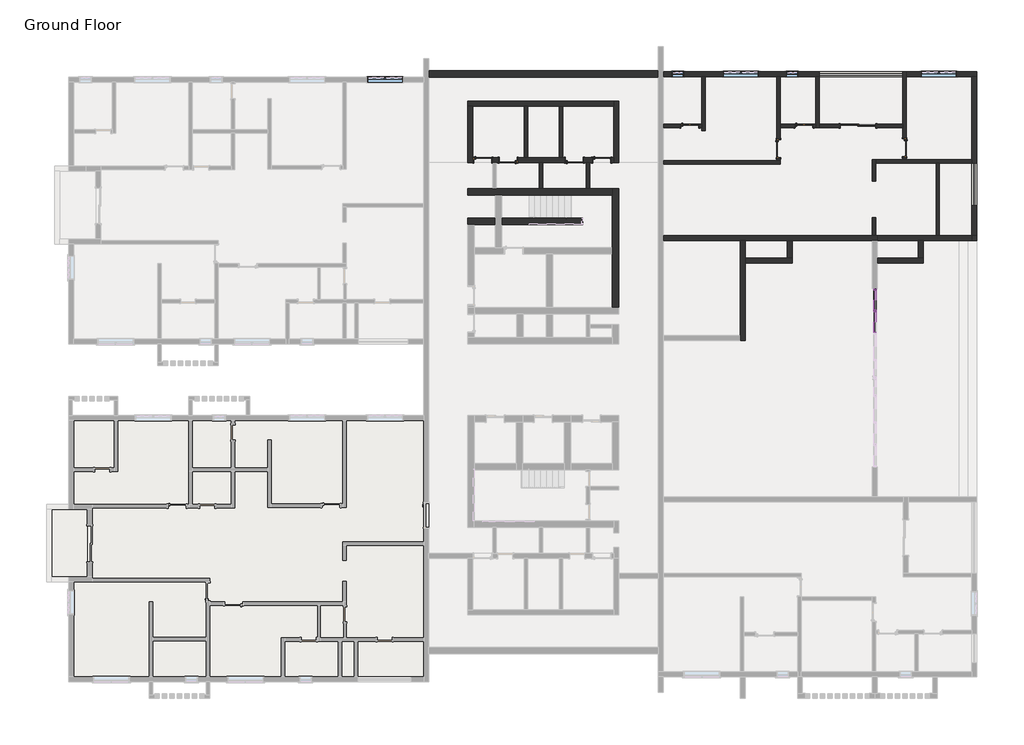
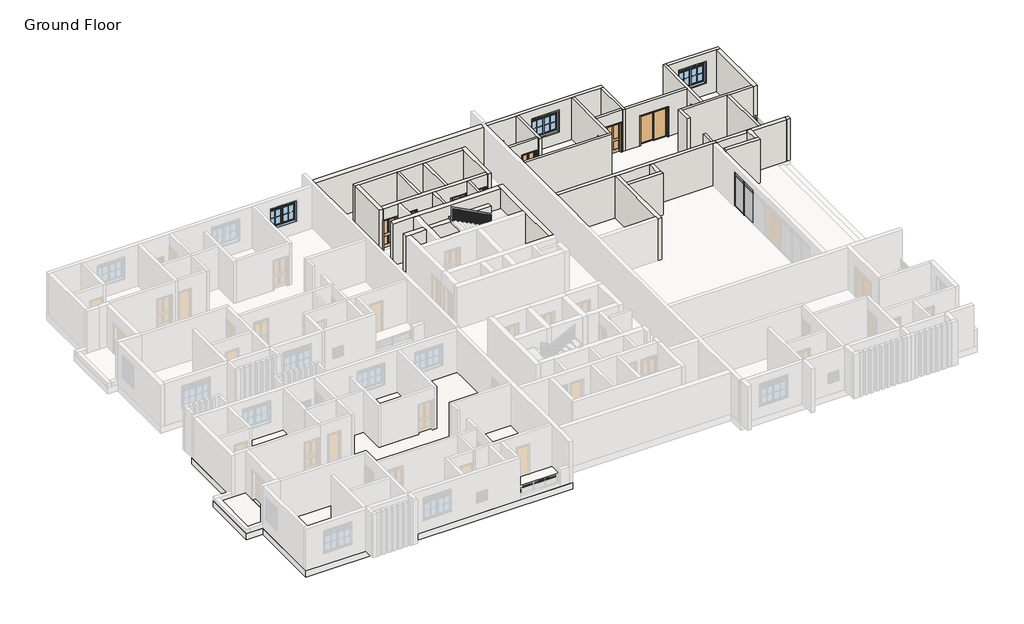
# One storey, part 5 of 9: 38 walls, 9 doors, 9 members, 5 windows, 4 plates, 2 slabs.
"""IFC4 building model written with IfcOpenShell, lengths in millimetres."""

from ifc_helpers import new_model, si_unit, frame, origin, origin_with_axes, place, context, project, spatial, polyline, outline, extrude, faceted_brep, transform, mapped, element, save
from components import door_double_sliding_6_85a7ba4d, door_interior_single_4_panel_wood_3_x_7_bed_room_doors_9f8eaeea, door_interior_single_4_panel_wood_3_x_7_bed_room_doors_167030f9, door_interior_single_4_panel_wood_3_x_7_bed_room_doors_330f8e7c, door_interior_single_4_panel_wood_3_x_7_bed_room_doors_7969a7cd, member_75d1e245, member_bf0a6844, member_74e81316, member_697f972d, member_78934672, member_3c3dc66a, member_222163d1, member_860c46db, system_panel_glazed_1d13bf28, system_panel_glazed_6ba3ac31, system_panel_glazed_eda788cd, system_panel_glazed_98578528, window_casement_double_awning_double_6_x_5_2a8633dc, window_double_hung_d0105baa

model = new_model("IFC4")

# Units and contexts
model_context = context("Model", 3, world=origin())
ifc_project = project(units=[si_unit("LENGTHUNIT", "METRE", prefix="MILLI")], contexts=[model_context])

# Site, building, storey
site = spatial("IfcSite", under=ifc_project)
building = spatial("IfcBuilding", under=site)
storey = spatial("IfcBuildingStorey", under=building, Name="Ground Floor", Elevation=0.0)

# Doors
placement = place(None, origin())
door_double_sliding_6_shape = door_double_sliding_6_85a7ba4d(model_context)
element("IfcDoor", 1, ObjectType="Door-Double-Sliding : 6'", at=placement, inside=storey, context=model_context, shape_type="MappedRepresentation", body=[
    mapped(door_double_sliding_6_shape, transform((26006.4546318, 26335.734892, 0.0), x_axis=(1.0, 0.0, 0.0), y_axis=(0.0, 1.0, 0.0), z_axis=(0.0, 0.0, 1.0))),
])
door_interior_single_4_panel_wood_3_x_7_bed_room_doors_shape = door_interior_single_4_panel_wood_3_x_7_bed_room_doors_9f8eaeea(model_context)
element("IfcDoor", 2, ObjectType="Door-Interior-Single-4_Panel-Wood : 3' x 7' Bed Room Doors", at=placement, inside=storey, context=model_context, shape_type="MappedRepresentation", body=[
    mapped(door_interior_single_4_panel_wood_3_x_7_bed_room_doors_shape, transform((17395.8546318, 26465.909892, 0.0), x_axis=(1.0, 0.0, 0.0), y_axis=(0.0, 1.0, 0.0), z_axis=(0.0, 0.0, 1.0))),
])
element("IfcDoor", 3, ObjectType="Door-Interior-Single-4_Panel-Wood : 3' x 7' Bed Room Doors", at=placement, inside=storey, context=model_context, shape_type="MappedRepresentation", body=[
    mapped(door_interior_single_4_panel_wood_3_x_7_bed_room_doors_shape, transform((23237.8546318, 26465.909892, 0.0), x_axis=(1.0, 0.0, 0.0), y_axis=(0.0, 1.0, 0.0), z_axis=(0.0, 0.0, 1.0))),
])
element("IfcDoor", 4, ObjectType="Door-Interior-Single-4_Panel-Wood : 3' x 7' Bed Room Doors", at=placement, inside=storey, context=model_context, shape_type="MappedRepresentation", body=[
    mapped(door_interior_single_4_panel_wood_3_x_7_bed_room_doors_shape, transform((28384.5296318, 25357.834892, 0.0), x_axis=(0.0, -1.0, 0.0), y_axis=(1.0, 0.0, 0.0), z_axis=(0.0, 0.0, 1.0))),
])
door_interior_single_4_panel_wood_3_x_7_bed_room_doors_2_shape = door_interior_single_4_panel_wood_3_x_7_bed_room_doors_167030f9(model_context)
element("IfcDoor", 5, ObjectType="Door-Interior-Single-4_Panel-Wood : 3' x 7' Bed Room Doors", at=placement, inside=storey, context=model_context, shape_type="MappedRepresentation", body=[
    mapped(door_interior_single_4_panel_wood_3_x_7_bed_room_doors_2_shape, transform((21926.5796318, 25307.034892, 0.0), x_axis=(0.0, -1.0, 0.0), y_axis=(1.0, 0.0, 0.0), z_axis=(0.0, 0.0, 1.0))),
])
door_interior_single_4_panel_wood_3_x_7_bed_room_doors_3_shape = door_interior_single_4_panel_wood_3_x_7_bed_room_doors_330f8e7c(model_context)
element("IfcDoor", 6, ObjectType="Door-Interior-Single-4_Panel-Wood : 3' x 7' Bed Room Doors", at=placement, inside=storey, context=model_context, shape_type="MappedRepresentation", body=[
    mapped(door_interior_single_4_panel_wood_3_x_7_bed_room_doors_3_shape, transform((8099.4546318, 24719.659892, 0.0), x_axis=(-1.0, 0.0, 0.0), y_axis=(0.0, -1.0, 0.0), z_axis=(0.0, 0.0, 1.0))),
])
element("IfcDoor", 7, ObjectType="Door-Interior-Single-4_Panel-Wood : 3' x 7' Bed Room Doors", at=placement, inside=storey, context=model_context, shape_type="MappedRepresentation", body=[
    mapped(door_interior_single_4_panel_wood_3_x_7_bed_room_doors_3_shape, transform((6804.0546318, 24726.009892, 0.0), x_axis=(1.0, 0.0, 0.0), y_axis=(0.0, 1.0, 0.0), z_axis=(0.0, 0.0, 1.0))),
])
element("IfcDoor", 8, ObjectType="Door-Interior-Single-4_Panel-Wood : 3' x 7' Bed Room Doors", at=placement, inside=storey, context=model_context, shape_type="MappedRepresentation", body=[
    mapped(door_interior_single_4_panel_wood_3_x_7_bed_room_doors_3_shape, transform((12887.3546318, 24726.009892, 0.0), x_axis=(1.0, 0.0, 0.0), y_axis=(0.0, 1.0, 0.0), z_axis=(0.0, 0.0, 1.0))),
])
door_interior_single_4_panel_wood_3_x_7_bed_room_doors_4_shape = door_interior_single_4_panel_wood_3_x_7_bed_room_doors_7969a7cd(model_context)
element("IfcDoor", 9, ObjectType="Door-Interior-Single-4_Panel-Wood : 3' x 7' Bed Room Doors", at=placement, inside=storey, context=model_context, shape_type="MappedRepresentation", body=[
    mapped(door_interior_single_4_panel_wood_3_x_7_bed_room_doors_4_shape, transform((11490.3546318, 24719.659892, 0.0), x_axis=(1.0, 0.0, 0.0), y_axis=(0.0, 1.0, 0.0), z_axis=(0.0, 0.0, 1.0))),
])

# Members
member_shape = member_75d1e245(model_context)
element("IfcMember", 10, ObjectType="Rectangular Mullion : 2.5\" x 5\" rectangular", at=placement, inside=storey, context=model_context, shape_type="MappedRepresentation", body=[
    mapped(member_shape, transform((26870.0546318, 17001.234892, 2286.0), x_axis=(0.0, 1.0, 0.0), y_axis=(1.0, 0.0, 0.0), z_axis=(0.0, 0.0, -1.0))),
])
member_2_shape = member_bf0a6844(model_context)
element("IfcMember", 11, ObjectType="Rectangular Mullion : 2.5\" x 5\" rectangular", at=placement, inside=storey, context=model_context, shape_type="MappedRepresentation", body=[
    mapped(member_2_shape, transform((26870.0546318, 16969.484892, 2286.0), x_axis=(0.0, 0.0, 1.0), y_axis=(1.0, 0.0, 0.0), z_axis=(0.0, 1.0, 0.0))),
])
member_3_shape = member_74e81316(model_context)
element("IfcMember", 12, ObjectType="Rectangular Mullion : 2.5\" x 5\" rectangular", at=placement, inside=storey, context=model_context, shape_type="MappedRepresentation", body=[
    mapped(member_3_shape, transform((26870.0546318, 16969.484892, 2590.8), x_axis=(0.0, 0.0, 1.0), y_axis=(1.0, 0.0, 0.0), z_axis=(0.0, 1.0, 0.0))),
])
member_4_shape = member_697f972d(model_context)
element("IfcMember", 13, ObjectType="Rectangular Mullion : 2.5\" x 5\" rectangular", at=placement, inside=storey, context=model_context, shape_type="MappedRepresentation", body=[
    mapped(member_4_shape, transform((26870.0546318, 18080.734892, 2286.0), x_axis=(0.0, 0.0, 1.0), y_axis=(1.0, 0.0, 0.0), z_axis=(0.0, 1.0, 0.0))),
])
member_5_shape = member_78934672(model_context)
element("IfcMember", 14, ObjectType="Rectangular Mullion : 2.5\" x 5\" rectangular", at=placement, inside=storey, context=model_context, shape_type="MappedRepresentation", body=[
    mapped(member_5_shape, transform((26870.0546318, 18080.734892, 2590.8), x_axis=(0.0, 0.0, 1.0), y_axis=(1.0, 0.0, 0.0), z_axis=(0.0, 1.0, 0.0))),
])
member_6_shape = member_3c3dc66a(model_context)
element("IfcMember", 15, ObjectType="Rectangular Mullion : 2.5\" x 5\" rectangular", at=placement, inside=storey, context=model_context, shape_type="MappedRepresentation", body=[
    mapped(member_6_shape, transform((26870.0546318, 18144.234892, 2286.0), x_axis=(0.0, 1.0, 0.0), y_axis=(1.0, 0.0, 0.0), z_axis=(0.0, 0.0, -1.0))),
])
member_7_shape = member_222163d1(model_context)
element("IfcMember", 16, ObjectType="Rectangular Mullion : 2.5\" x 5\" rectangular", at=placement, inside=storey, context=model_context, shape_type="MappedRepresentation", body=[
    mapped(member_7_shape, transform((26870.0546318, 17001.234892, 0.0), x_axis=(0.0, 1.0, 0.0), y_axis=(1.0, 0.0, 0.0), z_axis=(0.0, 0.0, -1.0))),
])
element("IfcMember", 17, ObjectType="Rectangular Mullion : 2.5\" x 5\" rectangular", at=placement, inside=storey, context=model_context, shape_type="MappedRepresentation", body=[
    mapped(member_5_shape, transform((26870.0546318, 17032.984892, 0.0), x_axis=(0.0, 0.0, -1.0), y_axis=(1.0, 0.0, 0.0), z_axis=(0.0, -1.0, 0.0))),
])
member_8_shape = member_860c46db(model_context)
element("IfcMember", 18, ObjectType="Rectangular Mullion : 2.5\" x 5\" rectangular", at=placement, inside=storey, context=model_context, shape_type="MappedRepresentation", body=[
    mapped(member_8_shape, transform((26870.0546318, 18144.234892, 0.0), x_axis=(0.0, 1.0, 0.0), y_axis=(1.0, 0.0, 0.0), z_axis=(0.0, 0.0, -1.0))),
])

# Plates
system_panel_glazed_shape = system_panel_glazed_1d13bf28(model_context)
element("IfcPlate", 19, ObjectType="System Panel : Glazed", at=placement, inside=storey, context=model_context, shape_type="MappedRepresentation", body=[
    mapped(system_panel_glazed_shape, transform((26870.0546318, 16429.734892, 2317.75), x_axis=(0.0, 1.0, 0.0), y_axis=(-1.0, 0.0, 0.0), z_axis=(0.0, 0.0, 1.0))),
])
system_panel_glazed_2_shape = system_panel_glazed_6ba3ac31(model_context)
element("IfcPlate", 20, ObjectType="System Panel : Glazed", at=placement, inside=storey, context=model_context, shape_type="MappedRepresentation", body=[
    mapped(system_panel_glazed_2_shape, transform((26870.0546318, 17556.859892, 2317.75), x_axis=(0.0, 1.0, 0.0), y_axis=(-1.0, 0.0, 0.0), z_axis=(0.0, 0.0, 1.0))),
])
system_panel_glazed_3_shape = system_panel_glazed_eda788cd(model_context)
element("IfcPlate", 21, ObjectType="System Panel : Glazed", at=placement, inside=storey, context=model_context, shape_type="MappedRepresentation", body=[
    mapped(system_panel_glazed_3_shape, transform((26870.0546318, 17556.859892, 63.5), x_axis=(0.0, 1.0, 0.0), y_axis=(-1.0, 0.0, 0.0), z_axis=(0.0, 0.0, 1.0))),
])
system_panel_glazed_4_shape = system_panel_glazed_98578528(model_context)
element("IfcPlate", 22, ObjectType="System Panel : Glazed", at=placement, inside=storey, context=model_context, shape_type="MappedRepresentation", body=[
    mapped(system_panel_glazed_4_shape, transform((26870.0546318, 16429.734892, 63.5), x_axis=(0.0, 1.0, 0.0), y_axis=(-1.0, 0.0, 0.0), z_axis=(0.0, 0.0, 1.0))),
])

# Slabs
element("IfcSlab", 23, ObjectType="Deck", at=placement, inside=storey, context=model_context, shape_type="Brep", body=[
    faceted_brep([(-14392.2453682, 7095.234892, -457.2), (-14392.2453682, 6841.234892, -457.2), (-13439.7453682, 6841.234892, -457.2), (-13439.7453682, 3386.834892, -457.2), (-14392.2453682, 3386.834892, -457.2), (-14392.2453682, 3132.834892, -457.2), (-15522.5453682, 3132.834892, -457.2), (-15522.5453682, 7095.234892, -457.2), (-14392.2453682, 7095.234892, 0.0), (-15522.5453682, 7095.234892, 0.0), (-15522.5453682, 6841.234892, 0.0), (-15522.5453682, 3132.834892, 0.0), (-15268.5453682, 3132.834892, 0.0), (-14392.2453682, 3132.834892, 0.0), (-14392.2453682, 3386.834892, 0.0), (-13439.7453682, 3386.834892, 0.0), (-13439.7453682, 6841.234892, 0.0), (-14392.2453682, 6841.234892, 0.0)], [[[0, 1, 2, 3, 4, 5, 6, 7]], [[8, 9, 10, 11, 12, 13, 14, 15, 16, 17]], [[1, 0, 8, 17]], [[2, 1, 17, 16]], [[3, 2, 16, 15]], [[4, 3, 15, 14]], [[5, 4, 14, 13]], [[6, 5, 13, 12, 11]], [[7, 6, 11, 10, 9]], [[0, 7, 9, 8]]]),
])
element("IfcSlab", 24, ObjectType="cream", at=placement, inside=storey, context=model_context, shape_type="Brep", body=[
    faceted_brep([(4035.4546318, 11641.834892, -457.2), (4035.4546318, -1997.965108, -457.2), (-14392.2453682, -1997.965108, -457.2), (-14392.2453682, 3386.834892, -457.2), (-13439.7453682, 3386.834892, -457.2), (-13439.7453682, 6841.234892, -457.2), (-14392.2453682, 6841.234892, -457.2), (-14392.2453682, 11641.834892, -457.2), (4035.4546318, 11641.834892, 0.0), (3781.4546318, 11641.834892, 0.0), (-14392.2453682, 11641.834892, 0.0), (-14392.2453682, 11387.834892, 0.0), (-14392.2453682, 6841.234892, 0.0), (-14138.2453682, 6841.234892, 0.0), (-13439.7453682, 6841.234892, 0.0), (-13439.7453682, 5990.334892, 0.0), (-13439.7453682, 4161.534892, 0.0), (-13439.7453682, 3386.834892, 0.0), (-14392.2453682, 3386.834892, 0.0), (-14392.2453682, 3132.834892, 0.0), (-14392.2453682, -1743.965108, 0.0), (-14392.2453682, -1997.965108, 0.0), (403.2546318, -1997.965108, 0.0), (3146.4546318, -1997.965108, 0.0), (3781.4546318, -1997.965108, 0.0), (4035.4546318, -1997.965108, 0.0), (4035.4546318, 5901.434892, 0.0), (4035.4546318, 7171.434892, 0.0)], [[[0, 1, 2, 3, 4, 5, 6, 7]], [[8, 9, 10, 11, 12, 13, 14, 15, 16, 17, 18, 19, 20, 21, 22, 23, 24, 25, 26, 27]], [[1, 0, 8, 27, 26, 25]], [[2, 1, 25, 24, 23, 22, 21]], [[3, 2, 21, 20, 19, 18]], [[4, 3, 18, 17]], [[5, 4, 17, 16, 15, 14]], [[6, 5, 14, 13, 12]], [[7, 6, 12, 11, 10]], [[0, 7, 10, 9, 8]]]),
])

# Walls
element("IfcWall", 25, ObjectType="12\" EXTERIOR WALL", at=placement, inside=storey, context=model_context, shape_type="Brep", body=[
    faceted_brep([(13763.6546318, 17179.034892, 0.0), (13763.6546318, 23249.634892, 0.0), (13763.6546318, 23249.634892, 3048.0), (13763.6546318, 17179.034892, 3048.0), (13433.4546318, 23249.634892, 0.0), (13433.4546318, 22919.434892, 0.0), (13433.4546318, 20252.434892, 0.0), (13433.4546318, 19922.234892, 0.0), (13433.4546318, 17179.034892, 0.0), (13433.4546318, 17179.034892, 3048.0), (13433.4546318, 20252.434892, 3048.0), (13433.4546318, 22919.434892, 3048.0), (13433.4546318, 23249.634892, 3048.0)], [[[0, 1, 2, 3]], [[4, 5, 6, 7, 8, 9, 10, 11, 12]], [[1, 0, 8, 7, 6, 5, 4]], [[8, 0, 3, 9]], [[1, 4, 12, 2]], [[3, 2, 12, 11, 10, 9]]]),
])
element("IfcWall", 26, ObjectType="12\" EXTERIOR WALL", at=placement, inside=storey, context=model_context, shape_type="Brep", body=[
    faceted_brep([(13433.4546318, 23249.634892, 0.0), (12265.0546318, 23249.634892, 0.0), (12087.2546318, 23249.634892, 0.0), (9877.4546318, 23249.634892, 0.0), (9699.6546318, 23249.634892, 0.0), (7489.8546318, 23249.634892, 0.0), (7312.0546318, 23249.634892, 0.0), (6042.0546318, 23249.634892, 0.0), (6042.0546318, 23249.634892, 3048.0), (7312.0546318, 23249.634892, 3048.0), (7489.8546318, 23249.634892, 3048.0), (9699.6546318, 23249.634892, 3048.0), (9877.4546318, 23249.634892, 3048.0), (12087.2546318, 23249.634892, 3048.0), (12265.0546318, 23249.634892, 3048.0), (13433.4546318, 23249.634892, 3048.0), (6042.0546318, 22919.434892, 0.0), (7439.0546318, 22919.434892, 0.0), (7769.2546318, 22919.434892, 0.0), (13433.4546318, 22919.434892, 0.0), (13433.4546318, 22919.434892, 3048.0), (9166.2546318, 22919.434892, 3048.0), (7769.2546318, 22919.434892, 3048.0), (7439.0546318, 22919.434892, 3048.0), (6042.0546318, 22919.434892, 3048.0)], [[[0, 1, 2, 3, 4, 5, 6, 7, 8, 9, 10, 11, 12, 13, 14, 15]], [[16, 17, 18, 19, 20, 21, 22, 23, 24]], [[7, 6, 5, 4, 3, 2, 1, 0, 19, 18, 17, 16]], [[7, 16, 24, 8]], [[19, 0, 15, 20]], [[15, 14, 13, 12, 11, 10, 9, 8, 24, 23, 22, 21, 20]]]),
])
element("IfcWall", 27, ObjectType="12\" EXTERIOR WALL", at=placement, inside=storey, context=model_context, shape_type="Brep", body=[
    faceted_brep([(4035.4546318, 28964.634892, 0.0), (15770.2546318, 28964.634892, 0.0), (15770.2546318, 28964.634892, 3048.0), (4035.4546318, 28964.634892, 3048.0), (15770.2546318, 29294.834892, 0.0), (4035.4546318, 29294.834892, 0.0), (4035.4546318, 29294.834892, 3048.0), (15770.2546318, 29294.834892, 3048.0), (15770.2546318, 29244.034892, 3048.0)], [[[0, 1, 2, 3]], [[4, 5, 6, 7]], [[1, 0, 5, 4]], [[5, 0, 3, 6]], [[1, 4, 7, 8, 2]], [[3, 2, 8, 7, 6]]]),
])
element("IfcWall", 28, ObjectType="12\" EXTERIOR WALL", at=placement, inside=storey, context=model_context, shape_type="Brep", body=[
    faceted_brep([(11909.4546318, 21751.034892, 3200.4), (11909.4546318, 21751.034892, 0.0), (7769.2546318, 21751.034892, 0.0), (7769.2546318, 21751.034892, 3048.0), (9166.2546318, 21751.034892, 3048.0), (9166.2546318, 21751.034892, 3200.4), (11909.4546318, 21420.834892, 0.0), (11909.4546318, 21420.834892, 3200.4), (9166.2546318, 21420.834892, 3200.4), (9166.2546318, 21420.834892, 3048.0), (7769.2546318, 21420.834892, 3048.0), (7769.2546318, 21420.834892, 0.0)], [[[0, 1, 2, 3, 4, 5]], [[6, 7, 8, 9, 10, 11]], [[1, 6, 11, 2]], [[7, 0, 5, 8]], [[1, 0, 7, 6]], [[9, 4, 3, 10]], [[4, 9, 8, 5]], [[3, 2, 11, 10]]]),
    faceted_brep([(6042.0546318, 21751.034892, 0.0), (6042.0546318, 21751.034892, 3048.0), (7439.0546318, 21751.034892, 3048.0), (7439.0546318, 21751.034892, 0.0), (6042.0546318, 21420.834892, 3048.0), (6042.0546318, 21420.834892, 0.0), (6372.2546318, 21420.834892, 0.0), (7439.0546318, 21420.834892, 0.0), (7439.0546318, 21420.834892, 3048.0), (6372.2546318, 21420.834892, 3048.0)], [[[0, 1, 2, 3]], [[4, 5, 6, 7, 8, 9]], [[5, 0, 3, 7, 6]], [[0, 5, 4, 1]], [[1, 4, 9, 8, 2]], [[3, 2, 8, 7]]]),
])
element("IfcWall", 29, ObjectType="6\" INTERIOR WALL", at=placement, inside=storey, context=model_context, shape_type="SweptSolid", body=[
    extrude(outline(polyline([(9877.4546318, 24595.834892), (9877.4546318, 23249.634892), (9699.6546318, 23249.634892), (9699.6546318, 24595.834892), (9877.4546318, 24595.834892)])), origin_with_axes(), (0.0, 0.0, 1.0), 3048.0),
])
element("IfcWall", 30, ObjectType="6\" INTERIOR WALL", at=placement, inside=storey, context=model_context, shape_type="SweptSolid", body=[
    extrude(outline(polyline([(12265.0546318, 24595.834892), (12265.0546318, 23249.634892), (12087.2546318, 23249.634892), (12087.2546318, 24595.834892), (12265.0546318, 24595.834892)])), origin_with_axes(), (0.0, 0.0, 1.0), 3048.0),
])
element("IfcWall", 31, ObjectType="6\" INTERIOR WALL", at=placement, inside=storey, context=model_context, shape_type="SweptSolid", body=[
    extrude(outline(polyline([(10715.6546318, 24849.834892), (10715.6546318, 27491.434892), (10893.4546318, 27491.434892), (10893.4546318, 24849.834892), (10715.6546318, 24849.834892)])), origin_with_axes(), (0.0, 0.0, 1.0), 3048.0),
])
element("IfcWall", 32, ObjectType="6\" INTERIOR WALL", at=placement, inside=storey, context=model_context, shape_type="SweptSolid", body=[
    extrude(outline(polyline([(9090.0546318, 27491.434892), (9090.0546318, 24849.834892), (8912.2546318, 24849.834892), (8912.2546318, 27491.434892), (9090.0546318, 27491.434892)])), origin_with_axes(), (0.0, 0.0, 1.0), 3048.0),
])
element("IfcWall", 33, ObjectType="6\" INTERIOR WALL", at=placement, inside=storey, context=model_context, shape_type="Brep", body=[
    faceted_brep([(16024.2546318, 24519.634892, 0.0), (22018.6546318, 24519.634892, 0.0), (22018.6546318, 24519.634892, 3048.0), (16024.2546318, 24519.634892, 3048.0), (22018.6546318, 24697.434892, 0.0), (21840.8546318, 24697.434892, 0.0), (16024.2546318, 24697.434892, 0.0), (16024.2546318, 24697.434892, 3048.0), (21840.8546318, 24697.434892, 3048.0), (22018.6546318, 24697.434892, 3048.0)], [[[0, 1, 2, 3]], [[4, 5, 6, 7, 8, 9]], [[1, 0, 6, 5, 4]], [[6, 0, 3, 7]], [[1, 4, 9, 2]], [[3, 2, 9, 8, 7]]]),
])
element("IfcWall", 34, ObjectType="6\" INTERIOR WALL", at=placement, inside=storey, context=model_context, shape_type="SweptSolid", body=[
    extrude(outline(polyline([(0.0, 17878.4546318), (0.0, 18005.4546318), (3048.0, 18005.4546318), (3048.0, 16024.2546318), (0.0, 16024.2546318), (0.0, 16913.2546318), (2159.0, 16913.2546318), (2159.0, 17878.4546318), (0.0, 17878.4546318)])), frame((0.0, 26373.834892, 0.0), z_axis=(0.0, 1.0, 0.0), x_axis=(0.0, 0.0, 1.0)), (0.0, 0.0, 1.0), 177.8),
])
element("IfcWall", 35, ObjectType="6\" INTERIOR WALL", at=placement, inside=storey, context=model_context, shape_type="Brep", body=[
    faceted_brep([(18005.4546318, 28990.034892, 0.0), (18005.4546318, 26551.634892, 0.0), (18005.4546318, 26373.834892, 0.0), (18005.4546318, 26221.434892, 0.0), (18005.4546318, 26221.434892, 3048.0), (18005.4546318, 26373.834892, 3048.0), (18005.4546318, 26551.634892, 3048.0), (18005.4546318, 28990.034892, 3048.0), (18183.2546318, 26221.434892, 0.0), (18183.2546318, 28990.034892, 0.0), (18183.2546318, 28990.034892, 3048.0), (18183.2546318, 26221.434892, 3048.0)], [[[0, 1, 2, 3, 4, 5, 6, 7]], [[8, 9, 10, 11]], [[3, 2, 1, 0, 9, 8]], [[3, 8, 11, 4]], [[9, 0, 7, 10]], [[7, 6, 5, 4, 11, 10]]]),
])
element("IfcWall", 36, ObjectType="6\" INTERIOR WALL", at=placement, inside=storey, context=model_context, shape_type="Brep", body=[
    faceted_brep([(21840.8546318, 24824.434892, 0.0), (21840.8546318, 24697.434892, 0.0), (21840.8546318, 24697.434892, 3048.0), (21840.8546318, 28990.034892, 3048.0), (21840.8546318, 28990.034892, 0.0), (21840.8546318, 25789.634892, 0.0), (21840.8546318, 25789.634892, 2159.0), (21840.8546318, 24824.434892, 2159.0), (22018.6546318, 24697.434892, 0.0), (22018.6546318, 24824.434892, 0.0), (22018.6546318, 24824.434892, 2159.0), (22018.6546318, 25789.634892, 2159.0), (22018.6546318, 25789.634892, 0.0), (22018.6546318, 26373.834892, 0.0), (22018.6546318, 26551.634892, 0.0), (22018.6546318, 28990.034892, 0.0), (22018.6546318, 28990.034892, 3048.0), (22018.6546318, 26551.634892, 3048.0), (22018.6546318, 26373.834892, 3048.0), (22018.6546318, 24697.434892, 3048.0)], [[[0, 1, 2, 3, 4, 5, 6, 7]], [[8, 9, 10, 11, 12, 13, 14, 15, 16, 17, 18, 19]], [[4, 15, 14, 13, 12, 5]], [[8, 1, 0, 9]], [[15, 4, 3, 16]], [[1, 8, 19, 2]], [[3, 2, 19, 18, 17, 16]], [[7, 10, 9, 0]], [[10, 7, 6, 11]], [[11, 6, 5, 12]]]),
])
element("IfcWall", 37, ObjectType="6\" INTERIOR WALL", at=placement, inside=storey, context=model_context, shape_type="Brep", body=[
    faceted_brep([(23847.4546318, 28990.034892, 0.0), (23847.4546318, 26551.634892, 0.0), (23847.4546318, 26373.834892, 0.0), (23847.4546318, 26373.834892, 3048.0), (23847.4546318, 26551.634892, 3048.0), (23847.4546318, 28990.034892, 3048.0), (24025.2546318, 26373.834892, 0.0), (24025.2546318, 26551.634892, 0.0), (24025.2546318, 28990.034892, 0.0), (24025.2546318, 28990.034892, 3048.0), (24025.2546318, 26551.634892, 3048.0), (24025.2546318, 26373.834892, 3048.0)], [[[0, 1, 2, 3, 4, 5]], [[6, 7, 8, 9, 10, 11]], [[2, 1, 0, 8, 7, 6]], [[2, 6, 11, 3]], [[8, 0, 5, 9]], [[5, 4, 3, 11, 10, 9]]]),
])
element("IfcWall", 38, ObjectType="6\" INTERIOR WALL", at=placement, inside=storey, context=model_context, shape_type="SweptSolid", body=[
    extrude(outline(polyline([(0.0, 23720.4546318), (0.0, 23847.4546318), (3048.0, 23847.4546318), (3048.0, 22018.6546318), (0.0, 22018.6546318), (0.0, 22755.2546318), (2159.0, 22755.2546318), (2159.0, 23720.4546318), (0.0, 23720.4546318)])), frame((0.0, 26373.834892, 0.0), z_axis=(0.0, 1.0, 0.0), x_axis=(0.0, 0.0, 1.0)), (0.0, 0.0, 1.0), 177.8),
])
element("IfcWall", 39, ObjectType="6\" INTERIOR WALL", at=placement, inside=storey, context=model_context, shape_type="SweptSolid", body=[
    extrude(outline(polyline([(0.0, 25092.0546318), (2133.6, 25092.0546318), (2133.6, 26920.8546318), (0.0, 26920.8546318), (0.0, 28292.4546318), (3048.0, 28292.4546318), (3048.0, 24025.2546318), (0.0, 24025.2546318), (0.0, 25092.0546318)])), frame((0.0, 26373.834892, 0.0), z_axis=(0.0, 1.0, 0.0), x_axis=(0.0, 0.0, 1.0)), (0.0, 0.0, 1.0), 177.8),
])
element("IfcWall", 40, ObjectType="6\" INTERIOR WALL", at=placement, inside=storey, context=model_context, shape_type="Brep", body=[
    faceted_brep([(28470.2546318, 24748.234892, 0.0), (28470.2546318, 24875.234892, 0.0), (28470.2546318, 24875.234892, 2159.0), (28470.2546318, 25840.434892, 2159.0), (28470.2546318, 25840.434892, 0.0), (28470.2546318, 28990.034892, 0.0), (28470.2546318, 29244.034892, 0.0), (28470.2546318, 29244.034892, 3048.0), (28470.2546318, 28990.034892, 3048.0), (28470.2546318, 24748.234892, 3048.0), (28292.4546318, 24875.234892, 0.0), (28292.4546318, 24748.234892, 0.0), (28292.4546318, 24748.234892, 3048.0), (28292.4546318, 26373.834892, 3048.0), (28292.4546318, 26551.634892, 3048.0), (28292.4546318, 29244.034892, 3048.0), (28292.4546318, 29244.034892, 304.8), (28292.4546318, 29244.034892, 0.0), (28292.4546318, 28990.034892, 0.0), (28292.4546318, 26551.634892, 0.0), (28292.4546318, 26373.834892, 0.0), (28292.4546318, 25840.434892, 0.0), (28292.4546318, 25840.434892, 2159.0), (28292.4546318, 24875.234892, 2159.0)], [[[0, 1, 2, 3, 4, 5, 6, 7, 8, 9]], [[10, 11, 12, 13, 14, 15, 16, 17, 18, 19, 20, 21, 22, 23]], [[17, 6, 5, 4, 21, 20, 19, 18]], [[0, 11, 10, 1]], [[6, 17, 16, 15, 7]], [[9, 8, 7, 15, 14, 13, 12]], [[11, 0, 9, 12]], [[23, 2, 1, 10]], [[2, 23, 22, 3]], [[3, 22, 21, 4]]]),
])
element("IfcWall", 41, ObjectType="6\" INTERIOR WALL", at=placement, inside=storey, context=model_context, shape_type="Brep", body=[
    faceted_brep([(31823.0546318, 24748.234892, 0.0), (28470.2546318, 24748.234892, 0.0), (28292.4546318, 24748.234892, 0.0), (26920.8546318, 24748.234892, 0.0), (26920.8546318, 24748.234892, 3048.0), (28292.4546318, 24748.234892, 3048.0), (28470.2546318, 24748.234892, 3048.0), (31823.0546318, 24748.234892, 3048.0), (26920.8546318, 24570.434892, 0.0), (29994.2546318, 24570.434892, 0.0), (30172.0546318, 24570.434892, 0.0), (31823.0546318, 24570.434892, 0.0), (31823.0546318, 24570.434892, 3048.0), (30172.0546318, 24570.434892, 3048.0), (29994.2546318, 24570.434892, 3048.0), (26920.8546318, 24570.434892, 3048.0)], [[[0, 1, 2, 3, 4, 5, 6, 7]], [[8, 9, 10, 11, 12, 13, 14, 15]], [[3, 2, 1, 0, 11, 10, 9, 8]], [[3, 8, 15, 4]], [[7, 6, 5, 4, 15, 14, 13, 12]], [[11, 0, 7, 12]]]),
])
element("IfcWall", 42, ObjectType="6\" INTERIOR WALL", at=placement, inside=storey, context=model_context, shape_type="SweptSolid", body=[
    extrude(outline(polyline([(29994.2546318, 20862.034892), (29994.2546318, 24570.434892), (30172.0546318, 24570.434892), (30172.0546318, 20862.034892), (29994.2546318, 20862.034892)])), origin_with_axes(), (0.0, 0.0, 1.0), 3048.0),
])
element("IfcWall", 43, ObjectType="6\" INTERIOR WALL", at=placement, inside=storey, context=model_context, shape_type="Brep", body=[
    faceted_brep([(26743.0546318, 24748.234892, 0.0), (26743.0546318, 23656.034892, 0.0), (26743.0546318, 23656.034892, 3048.0), (26743.0546318, 24748.234892, 3048.0), (26920.8546318, 23656.034892, 0.0), (26920.8546318, 24570.434892, 0.0), (26920.8546318, 24748.234892, 0.0), (26920.8546318, 24748.234892, 3048.0), (26920.8546318, 24570.434892, 3048.0), (26920.8546318, 23656.034892, 3048.0)], [[[0, 1, 2, 3]], [[4, 5, 6, 7, 8, 9]], [[1, 0, 6, 5, 4]], [[1, 4, 9, 2]], [[6, 0, 3, 7]], [[3, 2, 9, 8, 7]]]),
])
element("IfcWall", 44, ObjectType="6\" INTERIOR WALL", at=placement, inside=storey, context=model_context, shape_type="SweptSolid", body=[
    extrude(outline(polyline([(26920.8546318, 21776.434892), (26920.8546318, 20862.034892), (26743.0546318, 20862.034892), (26743.0546318, 21776.434892), (26920.8546318, 21776.434892)])), origin_with_axes(), (0.0, 0.0, 1.0), 3048.0),
])
element("IfcWall", 45, ObjectType="9\" EXTERIOR WALL", at=placement, inside=storey, context=model_context, shape_type="Brep", body=[
    faceted_brep([(13763.6546318, 24595.834892, 0.0), (13763.6546318, 27745.434892, 0.0), (13763.6546318, 27745.434892, 3048.0), (13763.6546318, 24595.834892, 3048.0), (13509.6546318, 27745.434892, 0.0), (13509.6546318, 27491.434892, 0.0), (13509.6546318, 24849.834892, 0.0), (13509.6546318, 24595.834892, 0.0), (13509.6546318, 24595.834892, 3048.0), (13509.6546318, 27745.434892, 3048.0)], [[[0, 1, 2, 3]], [[4, 5, 6, 7, 8, 9]], [[1, 0, 7, 6, 5, 4]], [[1, 4, 9, 2]], [[7, 0, 3, 8]], [[3, 2, 9, 8]]]),
])
element("IfcWall", 46, ObjectType="9\" EXTERIOR WALL", at=placement, inside=storey, context=model_context, shape_type="Brep", body=[
    faceted_brep([(13509.6546318, 27745.434892, 0.0), (6042.0546318, 27745.434892, 0.0), (6042.0546318, 27745.434892, 3048.0), (13509.6546318, 27745.434892, 3048.0), (6042.0546318, 27491.434892, 0.0), (6296.0546318, 27491.434892, 0.0), (8912.2546318, 27491.434892, 0.0), (9090.0546318, 27491.434892, 0.0), (10715.6546318, 27491.434892, 0.0), (10893.4546318, 27491.434892, 0.0), (13509.6546318, 27491.434892, 0.0), (13509.6546318, 27491.434892, 3048.0), (6042.0546318, 27491.434892, 3048.0)], [[[0, 1, 2, 3]], [[4, 5, 6, 7, 8, 9, 10, 11, 12]], [[1, 0, 10, 9, 8, 7, 6, 5, 4]], [[10, 0, 3, 11]], [[1, 4, 12, 2]], [[3, 2, 12, 11]]]),
])
element("IfcWall", 47, ObjectType="9\" EXTERIOR WALL", at=placement, inside=storey, context=model_context, shape_type="Brep", body=[
    faceted_brep([(6296.0546318, 24595.834892, 0.0), (6296.0546318, 24849.834892, 0.0), (6296.0546318, 27491.434892, 0.0), (6296.0546318, 27491.434892, 3048.0), (6296.0546318, 24849.834892, 3048.0), (6296.0546318, 24595.834892, 3048.0), (6042.0546318, 27491.434892, 0.0), (6042.0546318, 24595.834892, 0.0), (6042.0546318, 24595.834892, 3048.0), (6042.0546318, 27491.434892, 3048.0)], [[[0, 1, 2, 3, 4, 5]], [[6, 7, 8, 9]], [[2, 1, 0, 7, 6]], [[2, 6, 9, 3]], [[7, 0, 5, 8]], [[5, 4, 3, 9, 8]]]),
])
element("IfcWall", 48, ObjectType="9\" EXTERIOR WALL", at=placement, inside=storey, context=model_context, shape_type="Brep", body=[
    faceted_brep([(7616.8546318, 24595.834892, 0.0), (7616.8546318, 24595.834892, 2159.0), (8582.0546318, 24595.834892, 2159.0), (8582.0546318, 24595.834892, 0.0), (9699.6546318, 24595.834892, 0.0), (9877.4546318, 24595.834892, 0.0), (11007.7546318, 24595.834892, 0.0), (11007.7546318, 24595.834892, 2159.0), (11972.9546318, 24595.834892, 2159.0), (11972.9546318, 24595.834892, 0.0), (12087.2546318, 24595.834892, 0.0), (12265.0546318, 24595.834892, 0.0), (12404.7546318, 24595.834892, 0.0), (12404.7546318, 24595.834892, 2159.0), (13369.9546318, 24595.834892, 2159.0), (13369.9546318, 24595.834892, 0.0), (13509.6546318, 24595.834892, 0.0), (13509.6546318, 24595.834892, 3048.0), (12265.0546318, 24595.834892, 3048.0), (12087.2546318, 24595.834892, 3048.0), (9877.4546318, 24595.834892, 3048.0), (9699.6546318, 24595.834892, 3048.0), (7489.8546318, 24595.834892, 3048.0), (7312.0546318, 24595.834892, 3048.0), (6296.0546318, 24595.834892, 3048.0), (6296.0546318, 24595.834892, 0.0), (6321.4546318, 24595.834892, 0.0), (6321.4546318, 24595.834892, 2159.0), (7286.6546318, 24595.834892, 2159.0), (7286.6546318, 24595.834892, 0.0), (7312.0546318, 24595.834892, 0.0), (7489.8546318, 24595.834892, 0.0), (7616.8546318, 24849.834892, 2159.0), (7616.8546318, 24849.834892, 0.0), (7286.6546318, 24849.834892, 0.0), (7286.6546318, 24849.834892, 2159.0), (6321.4546318, 24849.834892, 2159.0), (6321.4546318, 24849.834892, 0.0), (6296.0546318, 24849.834892, 0.0), (6296.0546318, 24849.834892, 3048.0), (8912.2546318, 24849.834892, 3048.0), (9090.0546318, 24849.834892, 3048.0), (10715.6546318, 24849.834892, 3048.0), (10893.4546318, 24849.834892, 3048.0), (13509.6546318, 24849.834892, 3048.0), (13509.6546318, 24849.834892, 0.0), (13369.9546318, 24849.834892, 0.0), (13369.9546318, 24849.834892, 2159.0), (12404.7546318, 24849.834892, 2159.0), (12404.7546318, 24849.834892, 0.0), (11972.9546318, 24849.834892, 0.0), (11972.9546318, 24849.834892, 2159.0), (11007.7546318, 24849.834892, 2159.0), (11007.7546318, 24849.834892, 0.0), (10893.4546318, 24849.834892, 0.0), (10715.6546318, 24849.834892, 0.0), (9090.0546318, 24849.834892, 0.0), (8912.2546318, 24849.834892, 0.0), (8582.0546318, 24849.834892, 0.0), (8582.0546318, 24849.834892, 2159.0)], [[[0, 1, 2, 3, 4, 5, 6, 7, 8, 9, 10, 11, 12, 13, 14, 15, 16, 17, 18, 19, 20, 21, 22, 23, 24, 25, 26, 27, 28, 29, 30, 31]], [[32, 33, 34, 35, 36, 37, 38, 39, 40, 41, 42, 43, 44, 45, 46, 47, 48, 49, 50, 51, 52, 53, 54, 55, 56, 57, 58, 59]], [[25, 38, 37, 26]], [[45, 16, 15, 46]], [[33, 0, 31, 30, 29, 34]], [[3, 58, 57, 56, 55, 54, 53, 6, 5, 4]], [[9, 50, 49, 12, 11, 10]], [[16, 45, 44, 17]], [[38, 25, 24, 39]], [[24, 23, 22, 21, 20, 19, 18, 17, 44, 43, 42, 41, 40, 39]], [[32, 1, 0, 33]], [[1, 32, 59, 2]], [[2, 59, 58, 3]], [[8, 51, 50, 9]], [[51, 8, 7, 52]], [[52, 7, 6, 53]], [[28, 35, 34, 29]], [[35, 28, 27, 36]], [[36, 27, 26, 37]], [[14, 47, 46, 15]], [[47, 14, 13, 48]], [[48, 13, 12, 49]]]),
])
element("IfcWall", 49, ObjectType="9\" EXTERIOR WALL", at=placement, inside=storey, context=model_context, shape_type="Brep", body=[
    faceted_brep([(16024.2546318, 20608.034892, 0.0), (19986.6546318, 20608.034892, 0.0), (20240.6546318, 20608.034892, 0.0), (22374.2546318, 20608.034892, 0.0), (22628.2546318, 20608.034892, 0.0), (26743.0546318, 20608.034892, 0.0), (26997.0546318, 20608.034892, 0.0), (26997.0546318, 20608.034892, 3048.0), (26743.0546318, 20608.034892, 3048.0), (22628.2546318, 20608.034892, 3048.0), (22374.2546318, 20608.034892, 3048.0), (20240.6546318, 20608.034892, 3048.0), (19986.6546318, 20608.034892, 3048.0), (16024.2546318, 20608.034892, 3048.0), (26997.0546318, 20862.034892, 0.0), (26920.8546318, 20862.034892, 0.0), (26743.0546318, 20862.034892, 0.0), (16024.2546318, 20862.034892, 0.0), (16024.2546318, 20862.034892, 3048.0), (26743.0546318, 20862.034892, 3048.0), (26920.8546318, 20862.034892, 3048.0), (26997.0546318, 20862.034892, 3048.0)], [[[0, 1, 2, 3, 4, 5, 6, 7, 8, 9, 10, 11, 12, 13]], [[14, 15, 16, 17, 18, 19, 20, 21]], [[6, 5, 4, 3, 2, 1, 0, 17, 16, 15, 14]], [[17, 0, 13, 18]], [[6, 14, 21, 7]], [[13, 12, 11, 10, 9, 8, 7, 21, 20, 19, 18]]]),
])
element("IfcWall", 50, ObjectType="9\" EXTERIOR WALL", at=placement, inside=storey, context=model_context, shape_type="Brep", body=[
    faceted_brep([(19986.6546318, 20608.034892, 0.0), (19986.6546318, 15731.234892, 0.0), (19986.6546318, 15477.234892, 0.0), (19986.6546318, 15477.234892, 3048.0), (19986.6546318, 20608.034892, 3048.0), (20240.6546318, 15477.234892, 0.0), (20240.6546318, 19439.634892, 0.0), (20240.6546318, 19693.634892, 0.0), (20240.6546318, 20608.034892, 0.0), (20240.6546318, 20608.034892, 3048.0), (20240.6546318, 19693.634892, 3048.0), (20240.6546318, 19439.634892, 3048.0), (20240.6546318, 15477.234892, 3048.0)], [[[0, 1, 2, 3, 4]], [[5, 6, 7, 8, 9, 10, 11, 12]], [[2, 1, 0, 8, 7, 6, 5]], [[8, 0, 4, 9]], [[2, 5, 12, 3]], [[4, 3, 12, 11, 10, 9]]]),
])
element("IfcWall", 51, ObjectType="9\" EXTERIOR WALL", at=placement, inside=storey, context=model_context, shape_type="Brep", body=[
    faceted_brep([(20240.6546318, 19439.634892, 0.0), (22628.2546318, 19439.634892, 0.0), (22628.2546318, 19439.634892, 3048.0), (20240.6546318, 19439.634892, 3048.0), (22628.2546318, 19693.634892, 0.0), (22374.2546318, 19693.634892, 0.0), (20240.6546318, 19693.634892, 0.0), (20240.6546318, 19693.634892, 3048.0), (22628.2546318, 19693.634892, 3048.0)], [[[0, 1, 2, 3]], [[4, 5, 6, 7, 8]], [[1, 0, 6, 5, 4]], [[6, 0, 3, 7]], [[1, 4, 8, 2]], [[3, 2, 8, 7]]]),
])
element("IfcWall", 52, ObjectType="9\" EXTERIOR WALL", at=placement, inside=storey, context=model_context, shape_type="SweptSolid", body=[
    extrude(outline(polyline([(22628.2546318, 20608.034892), (22628.2546318, 19693.634892), (22374.2546318, 19693.634892), (22374.2546318, 20608.034892), (22628.2546318, 20608.034892)])), origin_with_axes(), (0.0, 0.0, 1.0), 3048.0),
])
element("IfcWall", 53, ObjectType="9\" EXTERIOR WALL", at=placement, inside=storey, context=model_context, shape_type="Brep", body=[
    faceted_brep([(26997.0546318, 19439.634892, 0.0), (29333.8546318, 19439.634892, 0.0), (29333.8546318, 19439.634892, 3200.4), (26997.0546318, 19439.634892, 3200.4), (26997.0546318, 19693.634892, 0.0), (26997.0546318, 19693.634892, 3200.4), (29079.8546318, 19693.634892, 3200.4), (29333.8546318, 19693.634892, 3200.4), (29333.8546318, 19693.634892, 0.0), (29079.8546318, 19693.634892, 0.0)], [[[0, 1, 2, 3]], [[4, 5, 6, 7, 8, 9]], [[1, 0, 4, 9, 8]], [[3, 2, 7, 6, 5]], [[2, 1, 8, 7]], [[0, 3, 5, 4]]]),
])
element("IfcWall", 54, ObjectType="9\" EXTERIOR WALL", at=placement, inside=storey, context=model_context, shape_type="SweptSolid", body=[
    extrude(outline(polyline([(29333.8546318, 20608.034892), (29333.8546318, 19693.634892), (29079.8546318, 19693.634892), (29079.8546318, 20608.034892), (29333.8546318, 20608.034892)])), origin_with_axes(), (0.0, 0.0, 1.0), 3200.4),
])
element("IfcWall", 55, ObjectType="9\" EXTERIOR WALL", at=placement, inside=storey, context=model_context, shape_type="Brep", body=[
    faceted_brep([(16024.2546318, 28990.034892, 0.0), (18005.4546318, 28990.034892, 0.0), (18183.2546318, 28990.034892, 0.0), (21840.8546318, 28990.034892, 0.0), (22018.6546318, 28990.034892, 0.0), (23847.4546318, 28990.034892, 0.0), (24025.2546318, 28990.034892, 0.0), (24025.2546318, 28990.034892, 304.8), (24025.2546318, 28990.034892, 3048.0), (23847.4546318, 28990.034892, 3048.0), (22018.6546318, 28990.034892, 3048.0), (21840.8546318, 28990.034892, 3048.0), (18183.2546318, 28990.034892, 3048.0), (18005.4546318, 28990.034892, 3048.0), (16024.2546318, 28990.034892, 3048.0), (20926.4546318, 28990.034892, 2438.4), (20926.4546318, 28990.034892, 914.4), (19097.6546318, 28990.034892, 914.4), (19097.6546318, 28990.034892, 2438.4), (22323.4546318, 28990.034892, 914.4), (22323.4546318, 28990.034892, 1524.0), (22933.0546318, 28990.034892, 1524.0), (22933.0546318, 28990.034892, 914.4), (16481.4546318, 28990.034892, 914.4), (16481.4546318, 28990.034892, 1524.0), (17091.0546318, 28990.034892, 1524.0), (17091.0546318, 28990.034892, 914.4), (24025.2546318, 29244.034892, 0.0), (16024.2546318, 29244.034892, 0.0), (16024.2546318, 29244.034892, 3048.0), (24025.2546318, 29244.034892, 3048.0), (24025.2546318, 29244.034892, 304.8), (20926.4546318, 29244.034892, 914.4), (20926.4546318, 29244.034892, 2438.4), (19097.6546318, 29244.034892, 2438.4), (19097.6546318, 29244.034892, 914.4), (22323.4546318, 29244.034892, 1524.0), (22323.4546318, 29244.034892, 914.4), (22933.0546318, 29244.034892, 914.4), (22933.0546318, 29244.034892, 1524.0), (16481.4546318, 29244.034892, 1524.0), (16481.4546318, 29244.034892, 914.4), (17091.0546318, 29244.034892, 914.4), (17091.0546318, 29244.034892, 1524.0)], [[[0, 1, 2, 3, 4, 5, 6, 7, 8, 9, 10, 11, 12, 13, 14], [15, 16, 17, 18], [19, 20, 21, 22], [23, 24, 25, 26]], [[27, 28, 29, 30, 31], [32, 33, 34, 35], [36, 37, 38, 39], [40, 41, 42, 43]], [[6, 5, 4, 3, 2, 1, 0, 28, 27]], [[28, 0, 14, 29]], [[6, 27, 31, 30, 8, 7]], [[14, 13, 12, 11, 10, 9, 8, 30, 29]], [[16, 15, 33, 32]], [[17, 16, 32, 35]], [[18, 17, 35, 34]], [[15, 18, 34, 33]], [[37, 36, 20, 19]], [[38, 37, 19, 22]], [[39, 38, 22, 21]], [[36, 39, 21, 20]], [[41, 40, 24, 23]], [[42, 41, 23, 26]], [[43, 42, 26, 25]], [[40, 43, 25, 24]]]),
])
element("IfcWall", 56, ObjectType="9\" EXTERIOR WALL", at=placement, inside=storey, context=model_context, shape_type="Brep", body=[
    faceted_brep([(28470.2546318, 28990.034892, 0.0), (31823.0546318, 28990.034892, 0.0), (32077.0546318, 28990.034892, 0.0), (32077.0546318, 28990.034892, 3048.0), (31823.0546318, 28990.034892, 3048.0), (28470.2546318, 28990.034892, 3048.0), (31061.0546318, 28990.034892, 2438.4), (31061.0546318, 28990.034892, 914.4), (29232.2546318, 28990.034892, 914.4), (29232.2546318, 28990.034892, 2438.4), (32077.0546318, 29244.034892, 0.0), (28470.2546318, 29244.034892, 0.0), (28470.2546318, 29244.034892, 3048.0), (32077.0546318, 29244.034892, 3048.0), (31061.0546318, 29244.034892, 914.4), (31061.0546318, 29244.034892, 2438.4), (29232.2546318, 29244.034892, 2438.4), (29232.2546318, 29244.034892, 914.4)], [[[0, 1, 2, 3, 4, 5], [6, 7, 8, 9]], [[10, 11, 12, 13], [14, 15, 16, 17]], [[2, 1, 0, 11, 10]], [[2, 10, 13, 3]], [[11, 0, 5, 12]], [[5, 4, 3, 13, 12]], [[7, 6, 15, 14]], [[8, 7, 14, 17]], [[9, 8, 17, 16]], [[6, 9, 16, 15]]]),
])
element("IfcWall", 57, ObjectType="9\" EXTERIOR WALL", at=placement, inside=storey, context=model_context, shape_type="Brep", body=[
    faceted_brep([(31823.0546318, 28990.034892, 0.0), (31823.0546318, 24748.234892, 0.0), (31823.0546318, 24570.434892, 0.0), (31823.0546318, 24570.434892, 304.8), (31823.0546318, 24570.434892, 3048.0), (31823.0546318, 24748.234892, 3048.0), (31823.0546318, 28990.034892, 3048.0), (32077.0546318, 24570.434892, 0.0), (32077.0546318, 28990.034892, 0.0), (32077.0546318, 28990.034892, 3048.0), (32077.0546318, 24570.434892, 3048.0), (32077.0546318, 24570.434892, 304.8)], [[[0, 1, 2, 3, 4, 5, 6]], [[7, 8, 9, 10, 11]], [[2, 1, 0, 8, 7]], [[2, 7, 11, 10, 4, 3]], [[8, 0, 6, 9]], [[6, 5, 4, 10, 9]]]),
])
element("IfcWall", 58, ObjectType="9\" EXTERIOR WALL", at=placement, inside=storey, context=model_context, shape_type="Brep", body=[
    faceted_brep([(31823.0546318, 20862.034892, 0.0), (30172.0546318, 20862.034892, 0.0), (29994.2546318, 20862.034892, 0.0), (26997.0546318, 20862.034892, 0.0), (26997.0546318, 20862.034892, 3048.0), (29994.2546318, 20862.034892, 3048.0), (30172.0546318, 20862.034892, 3048.0), (31823.0546318, 20862.034892, 3048.0), (26997.0546318, 20608.034892, 0.0), (29079.8546318, 20608.034892, 0.0), (29333.8546318, 20608.034892, 0.0), (31823.0546318, 20608.034892, 0.0), (31823.0546318, 20608.034892, 3048.0), (26997.0546318, 20608.034892, 3048.0)], [[[0, 1, 2, 3, 4, 5, 6, 7]], [[8, 9, 10, 11, 12, 13]], [[3, 2, 1, 0, 11, 10, 9, 8]], [[3, 8, 13, 4]], [[7, 6, 5, 4, 13, 12]], [[11, 0, 7, 12]]]),
])
element("IfcWall", 59, ObjectType="9\" EXTERIOR WALL", at=placement, inside=storey, context=model_context, shape_type="SweptSolid", body=[
    extrude(outline(polyline([(28292.4546318, 28990.034892), (24025.2546318, 28990.034892), (24025.2546318, 29244.034892), (28292.4546318, 29244.034892), (28292.4546318, 28990.034892)])), origin_with_axes(), (0.0, 0.0, 1.0), 304.8),
])
element("IfcWall", 60, ObjectType="9\" EXTERIOR WALL", at=placement, inside=storey, context=model_context, shape_type="Brep", body=[
    faceted_brep([(31823.0546318, 20862.034892, 0.0), (31823.0546318, 20608.034892, 0.0), (31823.0546318, 20608.034892, 3048.0), (31823.0546318, 20862.034892, 3048.0), (31823.0546318, 20862.034892, 1219.2), (32077.0546318, 20608.034892, 0.0), (32077.0546318, 20862.034892, 0.0), (32077.0546318, 20862.034892, 1219.2), (32077.0546318, 20862.034892, 3048.0), (32077.0546318, 20608.034892, 3048.0)], [[[0, 1, 2, 3, 4]], [[5, 6, 7, 8, 9]], [[1, 0, 6, 5]], [[6, 0, 4, 3, 8, 7]], [[1, 5, 9, 2]], [[3, 2, 9, 8]]]),
])
element("IfcWall", 61, ObjectType="9\" EXTERIOR WALL", at=placement, inside=storey, context=model_context, shape_type="Brep", body=[
    faceted_brep([(31823.0546318, 22386.034892, 0.0), (31823.0546318, 20862.034892, 0.0), (31823.0546318, 20862.034892, 1219.2), (31823.0546318, 22386.034892, 1219.2), (31823.0546318, 22386.034892, 304.8), (32077.0546318, 22386.034892, 0.0), (32077.0546318, 22386.034892, 304.8), (32077.0546318, 22386.034892, 1219.2), (32077.0546318, 20862.034892, 1219.2), (32077.0546318, 20862.034892, 0.0)], [[[0, 1, 2, 3, 4]], [[5, 6, 7, 8, 9]], [[1, 0, 5, 9]], [[3, 2, 8, 7]], [[0, 4, 3, 7, 6, 5]], [[2, 1, 9, 8]]]),
])
element("IfcWall", 62, ObjectType="9\" EXTERIOR WALL", at=placement, inside=storey, context=model_context, shape_type="SweptSolid", body=[
    extrude(outline(polyline([(31823.0546318, 22386.034892), (31823.0546318, 24570.434892), (32077.0546318, 24570.434892), (32077.0546318, 22386.034892), (31823.0546318, 22386.034892)])), origin_with_axes(), (0.0, 0.0, 1.0), 304.8),
])

# Windows
window_casement_double_awning_double_6_x_5_shape = window_casement_double_awning_double_6_x_5_2a8633dc(model_context)
element("IfcWindow", 63, ObjectType="Window-Casement-Double-Awning-Double : 6' x 5'", at=placement, inside=storey, context=model_context, shape_type="MappedRepresentation", body=[
    mapped(window_casement_double_awning_double_6_x_5_shape, transform((1800.2546318, 28837.634892, 0.0), x_axis=(1.0, 0.0, 0.0), y_axis=(0.0, 1.0, 0.0), z_axis=(0.0, 0.0, 1.0))),
])
element("IfcWindow", 64, ObjectType="Window-Casement-Double-Awning-Double : 6' x 5'", at=placement, inside=storey, context=model_context, shape_type="MappedRepresentation", body=[
    mapped(window_casement_double_awning_double_6_x_5_shape, transform((20012.0546318, 29117.034892, 0.0), x_axis=(1.0, 0.0, 0.0), y_axis=(0.0, 1.0, 0.0), z_axis=(0.0, 0.0, 1.0))),
])
element("IfcWindow", 65, ObjectType="Window-Casement-Double-Awning-Double : 6' x 5'", at=placement, inside=storey, context=model_context, shape_type="MappedRepresentation", body=[
    mapped(window_casement_double_awning_double_6_x_5_shape, transform((30146.6546318, 29117.034892, 0.0), x_axis=(1.0, 0.0, 0.0), y_axis=(0.0, 1.0, 0.0), z_axis=(0.0, 0.0, 1.0))),
])
window_double_hung_shape = window_double_hung_d0105baa(model_context)
element("IfcWindow", 66, ObjectType="Window-Double-Hung", at=placement, inside=storey, context=model_context, shape_type="MappedRepresentation", body=[
    mapped(window_double_hung_shape, transform((22628.2546318, 29117.034892, 0.0), x_axis=(1.0, 0.0, 0.0), y_axis=(0.0, 1.0, 0.0), z_axis=(0.0, 0.0, 1.0))),
])
element("IfcWindow", 67, ObjectType="Window-Double-Hung", at=placement, inside=storey, context=model_context, shape_type="MappedRepresentation", body=[
    mapped(window_double_hung_shape, transform((16786.2546318, 29117.034892, 0.0), x_axis=(1.0, 0.0, 0.0), y_axis=(0.0, 1.0, 0.0), z_axis=(0.0, 0.0, 1.0))),
])

save(model, "model.ifc")

# Revit data of these elements
# Type "Door-Double-Sliding : 6'"
#   Type Mark = "17"
#   Construction Type Id = "opn-d45"
#   Assembly Code = "C1020"
#   Analytic Construction = "Wood frame, double glass door "
#   Thickness = 0' - 2"
#   Thermal Resistance (R) = 1.8150 (h·ft²·°F)/BTU
#   Heat Transfer Coefficient (U) = 0.5510 BTU/(h·ft²·°F)
#   Height = 7' - 0"
#   Rail Width = 0' - 2"
#   Stiles = 0' - 2"
#   Trim Projection Ext = 0' - 1"
#   Trim Projection Int = 0' - 1"
#   Trim Width = 0' - 3"
#   Width = 6' - 0"
#   Define Thermal Properties by = 1
#   Glazing = Glass
#   Panel Material = Wood - Birch - Solid Stained Light Low Gloss
#   Trim Material = Paint - Sienna
#   Visual Light Transmittance = 0
#   Solar Heat Gain Coefficient = 0
#   Function = (empty or 0)
#   Wall Closure = (empty or 0)
# Type "Door-Interior-Single-4_Panel-Wood : 3' x 7' Bed Room Doors"
#   Type Mark = "13"
#   Assembly Code = "C1020300"
#   Analytic Construction = "Wooden"
#   Top Rail = 0' - 4 11/16"
#   Thickness = 0' - 1 3/8"
#   Thermal Resistance (R) = 2.5876 (h·ft²·°F)/BTU
#   Swing Angle [instance default] = 90.00°
#   Stiles = 0' - 2 3/8"
#   Rough Width = 3' - 2"
#   Rough Height = 7' - 1"
#   Mullion = 0' - 4 1/2"
#   Lock Rail = 0' - 7 1/2"
#   Height = 7' - 0"
#   Width = 3' - 0"
#   Heat Transfer Coefficient (U) = 0.3865 BTU/(h·ft²·°F)
#   Bottom Rail = 0' - 9 1/8"
#   Trim Material = Cherry
#   Panel Material = Cherry
#   Frame Material = Cherry
#   Door Handle Material = Aluminum
#   Visual Light Transmittance = 0
#   Solar Heat Gain Coefficient = 0
#   Wall Closure = (empty or 0)
#   Function = (empty or 0)
# Type "Rectangular Mullion : 2.5\" x 5\" rectangular"
#   built-in parameter 1007304 = 0.416667 (stored number, unit not read)
#   built-in parameter 1007301 = 0.104167 (stored number, unit not read)
#   built-in parameter 1007300 = 0.104167 (stored number, unit not read)
# Type "System Panel : Glazed"
#   Construction Type Id = "GSP4R"
#   Analytic Construction = "1/8 in Pilkington single glazing"
#   Visual Light Transmittance = 0.9
#   Solar Heat Gain Coefficient = 0.86
#   Heat Transfer Coefficient (U) = 1.18115 BTU/(h·ft²·°F)
#   Define Thermal Properties by = 1
# Type "Deck"
#   Assembly Code = "B1010"
#   Function = 0
#   Layers, outside or top first: 1' - 6" "0 deck(1)" (function 1)
# Type "cream"
#   Assembly Code = "B1010"
#   Function = 0
#   Layers, outside or top first: 1' - 6" "0 cream Floor" (function 1)
# Type "12\" EXTERIOR WALL"
#   Assembly Code = "B2010"
#   Layers, outside or top first: 0' - 0 1/2" "0 Cream" (function 1); 1' - 0" no material (function 1); 0' - 0 1/2" "0 Cream" (function 1)
# Type "6\" INTERIOR WALL"
#   Assembly Code = "B2010"
#   Layers, outside or top first: 0' - 0 1/2" "0 Cream" (function 1); 0' - 6" no material (function 1); 0' - 0 1/2" "0 Cream" (function 1)
# Type "9\" EXTERIOR WALL"
#   Assembly Code = "B2010"
#   Layers, outside or top first: 0' - 0 1/2" "0 Cream" (function 1); 0' - 9" no material (function 1); 0' - 0 1/2" "0 Cream" (function 1)
# Type "Window-Casement-Double-Awning-Double : 6' x 5'"
#   Type Mark = "22"
#   Fire Rating = "0.5h"
#   Assembly Code = "B2020100"
#   Analytic Construction = "Double glazing - domestic"
#   Window Inset [instance default] = 0' - 0"
#   Wall Thickness [instance default] = 0' - 6"
#   Interior Wall Closure [instance default] = 0' - 2 1/4"
#   Half Width = 3' - 0"
#   Visual Light Transmittance = 0.81
#   Transom Height = 1' - 0"
#   Thermal Resistance (R) = 1.8146 (h·ft²·°F)/BTU
#   Solar Heat Gain Coefficient = 0.76
#   Rough Width = 6' - 0 1/2"
#   Rough Height = 5' - 0 1/2"
#   Open Window Height = 4' - 0"
#   Frame Extension [instance default] = 0' - 0 1/4"
#   Height = 5' - 0"
#   Heat Transfer Coefficient (U) = 0.5511 BTU/(h·ft²·°F)
#   Exterior Wall Closure [instance default] = 0' - 1 1/4"
#   Extension Jamb [instance default] = 0' - 2 1/4"
#   Default Sill Height = 3' - 0"
#   Width = 6' - 0"
#   Top Muntin Visibility = yes
#   Bottom Muntin Visibility = yes
#   Interior Trim Visibility [instance default] = yes
#   Exterior Trim Visibility [instance default] = yes
#   Extension Jamb Visibility [instance default] = yes
#   Interior Trim Material = Wood - Stained
#   Muntin Pattern = Muntin Pattern_2x2 : Muntin Pattern_2x2
#   Interior Trim = Trim-Window-Interior-Flat : Picture Frame
#   Interior Frame Material = Wood - Stained
#   Glass Panel Material = Glass
#   Exterior Trim Material = Clad - White
#   Exterior Trim = Trim-Window-Exterior-Flat : with Sill
#   Exterior Frame Material = Clad - White
#   Wall Closure = (empty or 0)
# Type "Window-Double-Hung"
#   Type Mark = "20"
#   Fire Rating = "0.5h"
#   Construction Type Id = "DG-DR"
#   Assembly Code = "B2020100"
#   Analytic Construction = "Double glazing - domestic"
#   Wall Thickness [instance default] = 0' - 6"
#   Window Inset [instance default] = 0' - 0"
#   Visual Light Transmittance = 0.81
#   Thermal Resistance (R) = 1.8146 (h·ft²·°F)/BTU
#   Solar Heat Gain Coefficient = 0.76
#   Muntin Width = 1' - 6"
#   Muntin Height = 0' - 8 1/8"
#   Interior Wall Closure [instance default] = 0' - 1 1/2"
#   Rough Width = 2' - 0 1/2"
#   Rough Height = 2' - 0 1/2"
#   Frame Extension [instance default] = 0' - 1 1/4"
#   Exterior Wall Closure [instance default] = 0' - 0 1/2"
#   Extension Jamb [instance default] = 0' - 1 1/2"
#   Heat Transfer Coefficient (U) = 0.5511 BTU/(h·ft²·°F)
#   Height = 2' - 0"
#   Width = 2' - 0"
#   Top Muntin Visibility = yes
#   Indicator Visibility [instance default] = yes
#   Extension Jamb Visibility [instance default] = yes
#   Interior Trim Visibility [instance default] = yes
#   Exterior Trim Visibility [instance default] = yes
#   Define Thermal Properties by = 1
#   Bottom Muntin Visibility = yes
#   Muntin Pattern = Muntin Pattern_2x2 : Muntin Pattern_2x2
#   Interior Trim Material = Wood - Stained
#   Interior Trim = Trim-Window-Interior-Flat : Picture Frame
#   Exterior Trim Material = Clad - White
#   Exterior Trim = Trim-Window-Exterior-Flat : with Sill
#   Glass Panel Material = Glass
#   Exterior Frame Material = Clad - White
#   Interior Frame Material = Wood - Stained
#   Wall Closure = (empty or 0)
# Element 1 (IfcDoor, "Door-Double-Sliding : 6'")
#   Phase Created = New Construction
#   Materials on its faces: "Paint - Sienna", "Wood - Birch - Solid Stained Light Low Gloss", "Glass"
# Elements 2, 3, 4, 5, 6, 7, 8, 9 (IfcDoor, "Door-Interior-Single-4_Panel-Wood : 3' x 7' Bed Room Doors")
#   Swing Angle = 90.00°
#   Phase Created = New Construction
#   Materials on its faces: "Cherry", "Aluminum"
# Elements 10, 11, 12, 13, 14, 15, 16, 17, 18 (IfcMember, "Rectangular Mullion : 2.5\" x 5\" rectangular")
#   Phase Created = New Construction
#   Materials on its faces: "Aluminum"
# Elements 19, 20, 21, 22 (IfcPlate, "System Panel : Glazed")
#   Phase Created = New Construction
#   Materials on its faces: "Glass"
# Element 23 (IfcSlab, "Deck")
#   Height Offset From Level = 0' - 0"
#   Phase Created = New Construction
#   Materials on its faces: "0 deck(1)", "0 olive green"
# Element 24 (IfcSlab, "cream")
#   Height Offset From Level = 0' - 0"
#   Phase Created = New Construction
#   Materials on its faces: "0 cream Floor", "0 olive green"
# Element 25 (IfcWall, "12\" EXTERIOR WALL")
#   Top Offset = 0' - 0"
#   Base Offset = 0' - 0"
#   wall height = 10' - 6"
#   Phase Created = New Construction
#   Base Constraint = Ground Floor
#   Top Constraint = 1st Floor
#   Materials on its faces: "0 Cream", "Default Wall"
# Elements 26, 27, 28 (IfcWall, "12\" EXTERIOR WALL")
#   Top Offset = 0' - 0"
#   Base Offset = 0' - 0"
#   wall height = 10' - 6"
#   Phase Created = New Construction
#   Base Constraint = Ground Floor
#   Top Constraint = 1st Floor
#   Materials on its faces: "Default Wall", "0 Cream"
# Elements 29, 30, 31, 32, 34, 35, 36, 38, 39, 40, 41, 42, 44 (IfcWall, "6\" INTERIOR WALL")
#   Top Offset = 0' - 0"
#   Base Offset = 0' - 0"
#   wall height = 10' - 6"
#   Phase Created = New Construction
#   Base Constraint = Ground Floor
#   Top Constraint = 1st Floor
#   Materials on its faces: "Default Wall", "0 Cream"
# Elements 33, 37, 43 (IfcWall, "6\" INTERIOR WALL")
#   Top Offset = 0' - 0"
#   Base Offset = 0' - 0"
#   wall height = 10' - 6"
#   Phase Created = New Construction
#   Base Constraint = Ground Floor
#   Top Constraint = 1st Floor
#   Materials on its faces: "0 Cream", "Default Wall"
# Elements 45, 46, 47, 49, 50, 51, 53, 60 (IfcWall, "9\" EXTERIOR WALL")
#   Top Offset = 0' - 0"
#   Base Offset = 0' - 0"
#   wall height = 10' - 6"
#   Phase Created = New Construction
#   Base Constraint = Ground Floor
#   Top Constraint = 1st Floor
#   Materials on its faces: "0 Cream", "Default Wall"
# Elements 48, 52, 54, 55, 56, 57, 58 (IfcWall, "9\" EXTERIOR WALL")
#   Top Offset = 0' - 0"
#   Base Offset = 0' - 0"
#   wall height = 10' - 6"
#   Phase Created = New Construction
#   Base Constraint = Ground Floor
#   Top Constraint = 1st Floor
#   Materials on its faces: "Default Wall", "0 Cream"
